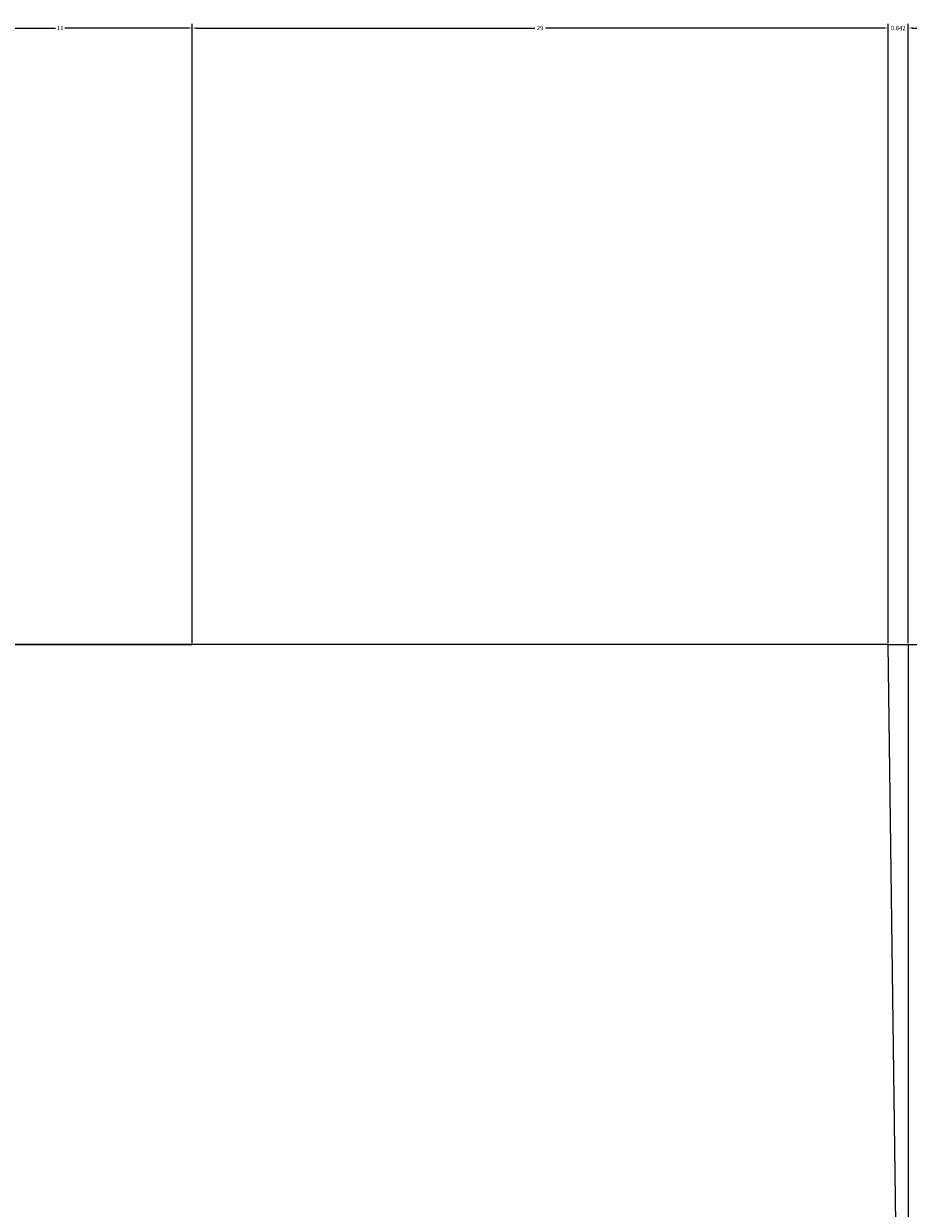
# Model space of a CAD drawing. Units: millimetres. Extents: x -136 to 10, y 158 to 257.
# Tile 3 of 6: x -99 to -62, y 208 to 257. Entities that reach past the tile are written whole.
import ezdxf

# ---------------------------------------------------------------- set-up
doc = ezdxf.new("R2010")
doc.units = ezdxf.units.MM
doc.layers.add('M-CONS', color=8, linetype='Continuous', lineweight=18)
doc.layers.add('M-DIMS', color=2, linetype='Continuous', lineweight=18)
doc.styles.get("Standard").update_dxf_attribs({"font": 'arial.ttf'})
doc.dimstyles.get("Standard").update_dxf_attribs({"dimtxt": 0.18, "dimasz": 0.18, "dimexe": 0.18, "dimexo": 0.0625, "dimgap": 0.09, "dimtad": 0, "dimtih": 1, "dimtoh": 1, "dimdec": 4, "dimzin": 0, "dimdsep": 46, "dimtxsty": 'Standard', "dimcen": 0.09, "dimadec": 0, "dimazin": 0, "dimtfac": 1, "dimtdec": 4, "dimtofl": 0, "dimtmove": 0, "dimatfit": 3, "dimfxl": 1, "dimtolj": 1, "dimtzin": 0, "dimarcsym": 0})

# ---------------------------------------------------------------- blocks, each defined once
blk = doc.blocks.new('*D1')
at = {"layer": 'Defpoints', "color": 0, "transparency": 16777216}
for p in [(-126, 231.107), (0, 231.107), (0, 158.407)]:
    blk.add_point(p, dxfattribs=at)
at = {"layer": 'M-DIMS', "color": 0, "lineweight": -2, "transparency": 16777216}
for p, q in [((-126, 231.044), (-126, 158.227)), ((0, 231.044), (0, 158.227)), ((-125.82, 158.407), (-63.28, 158.407)), ((-0.18, 158.407), (-62.72, 158.407))]:
    blk.add_line(p, q, dxfattribs=at)
at = {"layer": 'M-DIMS', "color": 0, "transparency": 16777216}
for points in [[(-125.82, 158.437), (-125.82, 158.377), (-126, 158.407)], [(-0.18, 158.437), (-0.18, 158.377), (0, 158.407)]]:
    blk.add_solid(points, dxfattribs=at)
at = {"layer": 'M-DIMS', "color": 0, "transparency": 16777216, "insert": (-63, 158.407), "char_height": 0.18, "attachment_point": 5}
blk.add_mtext('\\A1;126', dxfattribs=at)
blk = doc.blocks.new('*D3')
at = {"layer": 'Defpoints', "color": 0, "transparency": 16777216}
for p in [(-126, 231.107), (-135.7, 168.107), (-62.158, 168.107)]:
    blk.add_point(p, dxfattribs=at)
at = {"layer": 'M-DIMS', "color": 0, "lineweight": -2, "transparency": 16777216}
for p, q in [((-126.062, 231.107), (-135.88, 231.107)), ((-135.7, 230.927), (-135.7, 199.789)), ((-135.7, 168.287), (-135.7, 199.425)), ((-62.22, 168.107), (-135.88, 168.107))]:
    blk.add_line(p, q, dxfattribs=at)
at = {"layer": 'M-DIMS', "color": 0, "transparency": 16777216}
for points in [[(-135.73, 230.927), (-135.67, 230.927), (-135.7, 231.107)], [(-135.73, 168.287), (-135.67, 168.287), (-135.7, 168.107)]]:
    blk.add_solid(points, dxfattribs=at)
at = {"layer": 'M-DIMS', "color": 0, "transparency": 16777216, "insert": (-135.7, 199.607), "char_height": 0.18, "attachment_point": 5}
blk.add_mtext('\\A1;63', dxfattribs=at)
blk = doc.blocks.new('*D7')
at = {"layer": 'Defpoints', "color": 0, "transparency": 16777216}
for p in [(-92, 256.807), (-103, 231.107), (-92, 231.107)]:
    blk.add_point(p, dxfattribs=at)
at = {"layer": 'M-DIMS', "color": 0, "lineweight": -2, "transparency": 16777216}
for p, q in [((-103, 231.169), (-103, 256.987)), ((-102.82, 256.807), (-97.693, 256.807)), ((-92.18, 256.807), (-97.307, 256.807)), ((-92, 231.169), (-92, 256.987))]:
    blk.add_line(p, q, dxfattribs=at)
at = {"layer": 'M-DIMS', "color": 0, "transparency": 16777216}
for points in [[(-102.82, 256.837), (-102.82, 256.777), (-103, 256.807)], [(-92.18, 256.837), (-92.18, 256.777), (-92, 256.807)]]:
    blk.add_solid(points, dxfattribs=at)
at = {"layer": 'M-DIMS', "color": 0, "transparency": 16777216, "insert": (-97.5, 256.807), "char_height": 0.18, "attachment_point": 5}
blk.add_mtext('\\A1;11', dxfattribs=at)
blk = doc.blocks.new('*D8')
at = {"layer": 'Defpoints', "color": 0, "transparency": 16777216}
for p in [(-63, 256.807), (-92, 231.107), (-63, 231.107)]:
    blk.add_point(p, dxfattribs=at)
at = {"layer": 'M-DIMS', "color": 0, "lineweight": -2, "transparency": 16777216}
for p, q in [((-92, 231.169), (-92, 256.987)), ((-91.82, 256.807), (-77.721, 256.807)), ((-63.18, 256.807), (-77.279, 256.807)), ((-63, 231.169), (-63, 256.987))]:
    blk.add_line(p, q, dxfattribs=at)
at = {"layer": 'M-DIMS', "color": 0, "transparency": 16777216}
for points in [[(-91.82, 256.837), (-91.82, 256.777), (-92, 256.807)], [(-63.18, 256.837), (-63.18, 256.777), (-63, 256.807)]]:
    blk.add_solid(points, dxfattribs=at)
at = {"layer": 'M-DIMS', "color": 0, "transparency": 16777216, "insert": (-77.5, 256.807), "char_height": 0.18, "attachment_point": 5}
blk.add_mtext('\\A1;29', dxfattribs=at)
blk = doc.blocks.new('*D9')
at = {"layer": 'Defpoints', "color": 0, "transparency": 16777216}
for p in [(-62.157998, 256.806753), (-63, 231.106753), (-62.157998, 231.106753)]:
    blk.add_point(p, dxfattribs=at)
at = {"layer": 'M-DIMS', "color": 0, "lineweight": -2, "transparency": 16777216}
for p, q in [((-63.18, 256.806753), (-63.36, 256.806753)), ((-63, 231.169253), (-63, 256.986753)), ((-62.157998, 231.169253), (-62.157998, 256.986753)), ((-61.977998, 256.806753), (-61.797998, 256.806753))]:
    blk.add_line(p, q, dxfattribs=at)
at = {"layer": 'M-DIMS', "color": 0, "transparency": 16777216}
for points in [[(-63.18, 256.836753), (-63.18, 256.776753), (-63, 256.806753)], [(-61.977998, 256.836753), (-61.977998, 256.776753), (-62.157998, 256.806753)]]:
    blk.add_solid(points, dxfattribs=at)
at = {"layer": 'M-DIMS', "color": 0, "transparency": 16777216, "insert": (-62.578999, 256.806753), "char_height": 0.18, "attachment_point": 5}
blk.add_mtext('\\A1;0.842', dxfattribs=at)

msp = doc.modelspace()

# ---------------------------------------------------------------- linework, layer by layer
at = {"layer": 'M-CONS'}
for q in [(-94, 231.1068, 128.8035), (-32, 231.1068, 128.8035)]:
    msp.add_line((-63, 231.1068, 128.8035), q, dxfattribs=at)
msp.add_polyline3d([(-62.158, 168.1068, 112.8035), (-63, 231.1068, 68.8035), (-62.158, 231.1068, 112.8035)], close=True, dxfattribs=at)
at = {"layer": 'M-CONS', "extrusion": (0, -1, 0)}
msp.add_circle((-108, 98.8035, -231.1068), 16, dxfattribs=at)

# ---------------------------------------------------------------- dimensions: what is measured, and where the dimension line sits
at = {"layer": 'M-DIMS'}
for base, p1, p2, override, picture, middle in [((-92, 256.8068), (-103, 231.1068), (-92, 231.1068), {"dimdec": 0, "dimlfac": 1, "dimrnd": 0, "dimzin": 0, "dimdsep": 46, "dimlunit": 2}, '*D7', (-97.5, 256.8068)), ((-63, 256.8068), (-92, 231.1068), (-63, 231.1068), {"dimdec": 0, "dimlfac": 1, "dimrnd": 0, "dimzin": 0, "dimdsep": 46, "dimlunit": 2}, '*D8', (-77.5, 256.8068)), ((-62.158, 256.8068), (-63, 231.1068), (-62.158, 231.1068), {"dimdec": 3, "dimlfac": 1, "dimrnd": 0, "dimzin": 0, "dimdsep": 46, "dimlunit": 2}, '*D9', (-62.579, 256.8068)), ((0, 158.4068), (-126, 231.1068), (0, 231.1068), {"dimdec": 0, "dimlfac": 1, "dimrnd": 0, "dimzin": 0, "dimdsep": 46, "dimlunit": 2}, '*D1', (-63, 158.4068))]:
    dim = msp.add_linear_dim(base=base, p1=p1, p2=p2, dimstyle='Standard', override=override, dxfattribs=at)
    dim.commit()
    dim.dimension.update_dxf_attribs({"geometry": picture, "text_midpoint": middle})
dim = msp.add_linear_dim(base=(-135.7, 168.1068), p1=(-126, 231.1068), p2=(-62.158, 168.1068), angle=90, dimstyle='Standard', override={"dimdec": 0, "dimlfac": 1, "dimrnd": 0, "dimzin": 0, "dimdsep": 46, "dimlunit": 2}, dxfattribs=at)
dim.commit()
dim.dimension.update_dxf_attribs({"geometry": '*D3', "text_midpoint": (-135.7, 199.6068)})

doc.saveas('drawing.dxf')
